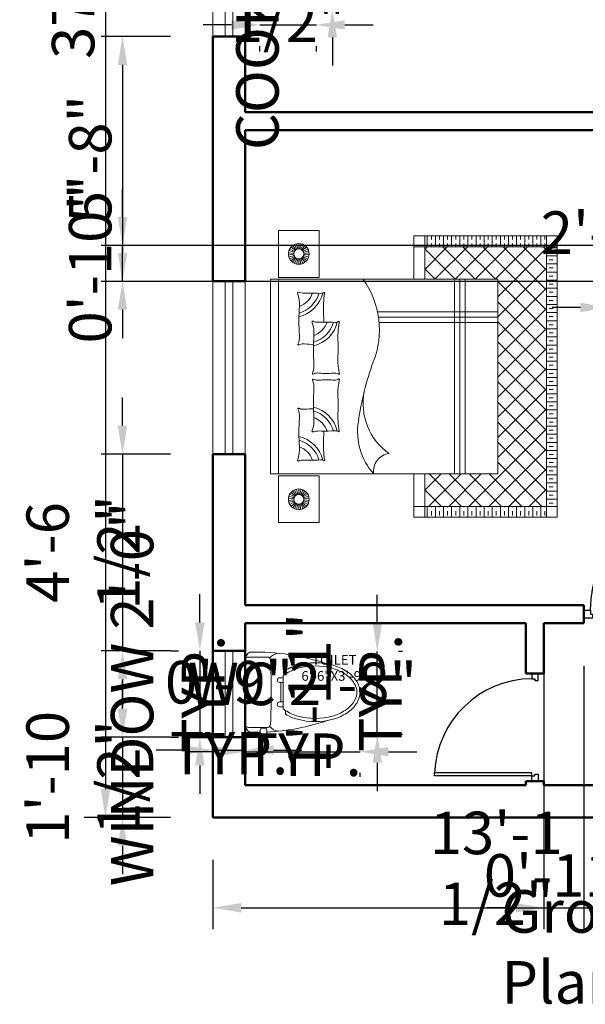
# Model space of a CAD drawing. Units: inches. Extents: x 314 to 688, y 344 to 882.
# Tile 1 of 3: x 314 to 471, y 344 to 618. Entities that reach past the tile are written whole.
import ezdxf

# ---------------------------------------------------------------- set-up
doc = ezdxf.new("R2010")
doc.units = ezdxf.units.IN
doc.header["$MEASUREMENT"] = 0
for name, color, linetype, lineweight in [('A-ANNO-TEXT', 7, 'Continuous', 25), ('A-AREA-IDEN', 7, 'Continuous', 25), ('A-DOOR', 4, 'Continuous', 25), ('A-FLOR-FIXT', 9, 'Continuous', 18), ('A-FURN', 8, 'Continuous', 18), ('WALL', 7, 'Continuous', 50), ('WINDOW', 2, 'Continuous', 18), ('YQ_DIM', 3, 'Continuous', 18)]:
    doc.layers.add(name, color=color, linetype=linetype, lineweight=lineweight)
doc.styles.add('YQ_DIM', font='SUPEROS.SHX', dxfattribs={"width": 0.8, "bigfont": 'HZDX.SHX'})
doc.dimstyles.new('yqi3_937', dxfattribs={"dimscale": 3.937008, "dimtxt": 3, "dimasz": 2, "dimexe": 1.5, "dimexo": 3, "dimgap": 0.5, "dimtad": 1, "dimdsep": 46, "dimlunit": 4, "dimtxsty": 'YQ_DIM', "dimcen": 0, "dimclrd": 256, "dimclre": 256, "dimclrt": 7, "dimadec": 1, "dimazin": 2, "dimtfac": 1, "dimtix": 1, "dimtmove": 2, "dimatfit": 2, "dimfxl": 1, "dimtolj": 1, "dimtzin": 0, "dimarcsym": 0})

# ---------------------------------------------------------------- blocks, each defined once
blk = doc.blocks.new('*D2')
at = {"layer": 'Defpoints', "color": 0, "transparency": 16777216}
for p in [(367.29, 840.23), (337.46, 396.23), (367.29, 396.23)]:
    blk.add_point(p, dxfattribs=at)
at = {"layer": 'YQ_DIM', "color": 0, "lineweight": -2, "transparency": 16777216}
for p, q in [((355.48, 840.23), (331.55, 840.23)), ((337.46, 832.36), (337.46, 404.11)), ((355.48, 396.23), (331.55, 396.23))]:
    blk.add_line(p, q, dxfattribs=at)
at = {"layer": 'YQ_DIM', "color": 0, "transparency": 16777216}
for points in [[(336.14, 832.36), (338.77, 832.36), (337.46, 840.23)], [(336.14, 404.11), (338.77, 404.11), (337.46, 396.23)]]:
    blk.add_solid(points, dxfattribs=at)
at = {"layer": 'YQ_DIM', "color": 0, "transparency": 16777216, "insert": (328.46, 618.23), "char_height": 11.811, "attachment_point": 5, "rotation": 90, "style": 'YQ_DIM'}
blk.add_mtext("\\A1;37'", dxfattribs=at)
blk = doc.blocks.new('DR_D01')
for p, q in [((-0.45, 0.93), (-0.42, 0.93)), ((-0.45, 0.03), (-0.45, 0.93)), ((-0.42, 0.03), (-0.42, 0.93)), ((-0.5, 0.03), (-0.42, 0.03)), ((-0.5, 0.03), (-0.5, -0.03)), ((-0.45, 0.03), (-0.45, 0)), ((-0.45, 0), (-0.435, 0)), ((-0.435, 0), (-0.435, -0.03)), ((0.435, 0), (0.435, -0.03)), ((0.45, 0), (0.435, 0)), ((0.45, 0.03), (0.45, 0)), ((0.5, 0.03), (0.45, 0.03)), ((0.5, -0.03), (0.5, 0.03)), ((-0.435, -0.03), (-0.5, -0.03)), ((0.435, -0.03), (0.5, -0.03))]:
    blk.add_line(p, q)
blk.add_arc((-0.4602, 0.0206), 0.9103, 0.59152, 87.46644)
blk = doc.blocks.new('WD_WIN4')
for p, q in [((-0.5, 0.5), (0.5, 0.5)), ((-0.5, 0.12), (0.5, 0.12)), ((-0.5, -0.12), (0.5, -0.12)), ((-0.5, -0.5), (0.5, -0.5))]:
    blk.add_line(p, q)
blk = doc.blocks.new('BED')
h = blk.add_hatch()
h.set_pattern_fill('TRANS', color=256, scale=12, style=0)
h.set_pattern_definition([(360, (4433.967, -9715.0492), (1e-15, 3), []), (360, (4433.967, -9713.5492), (1e-15, 3), [1.5, -1.5])])
h.paths.add_polyline_path([(48, -103), (52, -103), (52, -58), (48, -58)])
h.paths.add_polyline_path([(-48, -58), (-52, -58), (-52, -103), (-48, -103)])
h = blk.add_hatch()
h.set_pattern_fill('ANSI37', color=256, scale=42, angle=-90, style=0)
h.set_pattern_definition([(315, (7787.1367, 4477.8466), (3.7123106, 3.7123106), []), (45, (7787.1367, 4477.8466), (-3.7123106, 3.7123106), [])])
h.paths.add_polyline_path([(-36, -85), (-36, -58), (-48, -58), (-48, -103), (48, -103), (48, -58), (36, -58), (36, -85)])
h = blk.add_hatch()
h.set_pattern_fill('TRANS', color=256, scale=12, angle=-90, style=0)
h.set_pattern_definition([(270, (4433.967, -9715.0492), (3, -1e-15), []), (270, (4435.467, -9715.0492), (3, -1e-15), [1.5, -1.5])])
h.paths.add_polyline_path([(48, -107), (48, -103), (-48, -103), (-48, -107)])
for p, q in [((-36, -1), (36, -1)), ((-36, -85), (-36, -1)), ((36, -1), (36, -85)), ((-54, -4), (-54, -19)), ((-36.64, -4), (-54, -4)), ((-36.64, -4), (-36.64, -19)), ((-36, -4), (36, -4)), ((36.64, -4), (36.64, -19)), ((36.64, -4), (54, -4)), ((54, -4), (54, -19)), ((-47.19, -11.07), (-49.14, -10.66)), ((-47.07, -10.7), (-48.9, -9.89)), ((-46.88, -10.37), (-48.5, -9.2)), ((-46.62, -10.08), (-47.96, -8.6)), ((-46.31, -9.86), (-47.31, -8.13)), ((-45.96, -9.7), (-46.58, -7.8)), ((-45.58, -9.62), (-45.8, -7.63)), ((-45.2, -9.62), (-45, -7.63)), ((-44.82, -9.7), (-44.21, -7.79)), ((-44.47, -9.85), (-43.48, -8.12)), ((-44.16, -10.08), (-42.83, -8.59)), ((-43.9, -10.36), (-42.29, -9.18)), ((-43.71, -10.7), (-41.89, -9.88)), ((-43.59, -11.06), (-41.64, -10.64)), ((43.59, -11.06), (41.64, -10.64)), ((43.71, -10.7), (41.89, -9.88)), ((43.9, -10.36), (42.29, -9.18)), ((44.16, -10.08), (42.83, -8.59)), ((44.47, -9.85), (43.48, -8.12)), ((44.82, -9.7), (44.21, -7.79)), ((45.2, -9.62), (45, -7.63)), ((45.58, -9.62), (45.8, -7.63)), ((45.96, -9.7), (46.58, -7.8)), ((46.31, -9.86), (47.31, -8.13)), ((46.62, -10.08), (47.96, -8.6)), ((46.88, -10.37), (48.5, -9.2)), ((47.07, -10.7), (48.9, -9.89)), ((47.19, -11.07), (49.14, -10.66)), ((-47.23, -11.45), (-49.23, -11.45)), ((-47.19, -11.83), (-49.14, -12.25)), ((-47.07, -12.2), (-48.89, -13.01)), ((-46.87, -12.53), (-48.49, -13.71)), ((-46.62, -12.81), (-47.95, -14.3)), ((-46.3, -13.04), (-47.3, -14.77)), ((-45.95, -13.2), (-46.57, -15.1)), ((-45.58, -13.27), (-45.78, -15.26)), ((-45.19, -13.27), (-44.98, -15.26)), ((-44.82, -13.19), (-44.2, -15.09)), ((-44.47, -13.04), (-43.46, -14.77)), ((-44.16, -12.81), (-42.82, -14.29)), ((-43.9, -12.52), (-42.28, -13.7)), ((-43.71, -12.19), (-41.88, -13)), ((-43.59, -11.83), (-41.63, -12.24)), ((-43.55, -11.44), (-41.55, -11.44)), ((43.55, -11.44), (41.55, -11.44)), ((43.59, -11.83), (41.63, -12.24)), ((43.71, -12.19), (41.88, -13)), ((43.9, -12.52), (42.28, -13.7)), ((44.16, -12.81), (42.82, -14.29)), ((44.47, -13.04), (43.46, -14.77)), ((44.82, -13.19), (44.2, -15.09)), ((45.19, -13.27), (44.98, -15.26)), ((45.58, -13.27), (45.78, -15.26)), ((45.95, -13.2), (46.57, -15.1)), ((46.3, -13.04), (47.3, -14.77)), ((46.62, -12.81), (47.95, -14.3)), ((46.87, -12.53), (48.49, -13.71)), ((47.07, -12.2), (48.89, -13.01)), ((47.19, -11.83), (49.14, -12.25)), ((47.23, -11.45), (49.23, -11.45)), ((-36.64, -19), (-54, -19)), ((36.64, -19), (54, -19)), ((20, -85), (20, -41.14)), ((22, -85), (22, -40.91)), ((24, -85), (24, -40.55)), ((-52, -54), (-52, -107)), ((-52, -54), (-36, -54)), ((-48, -54), (-48, -107)), ((36, -54), (52, -54)), ((48, -54), (48, -107)), ((52, -54), (52, -107)), ((-52, -58), (-36, -58)), ((36, -58), (52, -58)), ((36, -69), (-36, -69)), ((36, -71), (-36, -71)), ((36, -73), (-36, -73)), ((36, -85), (-36, -85)), ((-52, -103), (52, -103)), ((-52, -107), (52, -107))]:
    blk.add_line(p, q)
for centre, radius in [((-45.39, -11.45), 3.84), ((-45.39, -11.45), 1.84), ((45.39, -11.45), 3.84), ((45.39, -11.45), 1.84)]:
    blk.add_circle(centre, radius)
for centre, radius, start, end in [((-30.92, -11.24), 0.328, 35.8976, 208.6272), ((30.92, -11.24), 0.328, 331.3728, 144.1024), ((-42.38, -17.5), 12.73, 27.1629, 28.6272), ((-44.37, -13.89), 13.5, 357.4804, 9.3956), ((10.15, -16.29), 41.07, 177.4804, 184.5075), ((-33.8, -8.61), 8.46, 289.8695, 338.9843), ((-33.8, -8.61), 12.06, 283.8498, 346.0842), ((-33.8, -8.61), 10.71, 286.0319, 344.1205), ((-26.84, 0.13), 11.82, 251.1782, 273.3982), ((-20.92, -99.64), 88.13, 86.2964, 93.3982), ((-14.79, -4.98), 6.73, 266.2964, 294.303), ((-8.24, -13.16), 3.86, 159.0146, 186.273), ((-36.64, -16.28), 24.71, 358.5721, 6.273), ((-11.92, -11.33), 0.242, 335.7259, 114.303), ((-5.69, -14.14), 6.59, 155.7259, 159.0146), ((11.92, -11.33), 0.242, 65.697, 204.2741), ((5.69, -14.14), 6.59, 20.9854, 24.2741), ((8.24, -13.16), 3.86, 353.727, 20.9854), ((36.64, -16.28), 24.71, 173.727, 181.4279), ((14.79, -4.98), 6.73, 245.697, 273.7036), ((20.92, -99.64), 88.13, 86.6018, 93.7036), ((33.8, -8.61), 12.06, 193.9158, 256.1502), ((33.8, -8.61), 10.71, 195.8795, 253.9681), ((33.8, -8.61), 8.46, 201.0157, 250.1305), ((26.84, 0.13), 11.82, 266.6018, 288.8218), ((-10.15, -16.29), 41.07, 355.4925, 2.5196), ((44.37, -13.89), 13.5, 170.6044, 182.5196), ((42.38, -17.5), 12.73, 151.3728, 152.8371), ((-20.16, -16.62), 0.328, 35.8976, 208.6272), ((-31.62, -22.87), 12.73, 27.1629, 28.6272), ((-33.61, -19.26), 13.5, 357.4804, 9.3956), ((-23.04, -13.99), 8.46, 289.8695, 338.9843), ((-23.04, -13.99), 12.06, 283.8498, 346.0842), ((-23.04, -13.99), 10.71, 286.0319, 344.1205), ((-16.08, -5.24), 11.82, 251.1782, 273.3982), ((-10.15, -105.01), 88.13, 86.2964, 93.3982), ((-4.03, -10.35), 6.73, 266.2964, 294.303), ((2.52, -18.53), 3.86, 159.0146, 186.273), ((-1.16, -16.7), 0.242, 335.7259, 114.303), ((5.07, -19.51), 6.59, 155.7259, 159.0146), ((1.16, -16.7), 0.242, 65.697, 204.2741), ((-5.07, -19.51), 6.59, 20.9854, 24.2741), ((-2.52, -18.53), 3.86, 353.727, 20.9854), ((4.03, -10.35), 6.73, 245.697, 273.7036), ((10.15, -105.01), 88.13, 86.6018, 93.7036), ((23.04, -13.99), 12.06, 193.9158, 256.1502), ((23.04, -13.99), 10.71, 195.8795, 253.9681), ((23.04, -13.99), 8.46, 201.0157, 250.1305), ((16.08, -5.24), 11.82, 266.6018, 288.8218), ((20.16, -16.62), 0.328, 331.3728, 144.1024), ((33.61, -19.26), 13.5, 170.6044, 182.5196), ((31.62, -22.87), 12.73, 151.3728, 152.8371), ((-30.88, -20.82), 0.25, 147.6219, 311.9343), ((-32.72, -19.65), 1.93, 327.6219, 339.2246), ((-32.67, -19.67), 1.88, 339.2246, 4.5075), ((-25.16, -53.53), 33, 93.5164, 99.6766), ((-25.27, -51.86), 31.33, 86.4836, 93.5164), ((-21.12, 15.68), 36.34, 266.4836, 271.5234), ((20.91, -21.66), 41.07, 177.4804, 184.5075), ((-25.88, -21.66), 24.71, 354.3784, 6.273), ((25.88, -21.66), 24.71, 173.727, 185.6216), ((-20.91, -21.66), 41.07, 355.4925, 2.5196), ((21.12, 15.68), 36.34, 268.4766, 273.5164), ((25.27, -51.86), 31.33, 86.4836, 93.5164), ((25.16, -53.53), 33, 80.3234, 86.4836), ((30.88, -20.82), 0.25, 228.0657, 32.3781), ((32.67, -19.67), 1.88, 175.4925, 200.7754), ((32.72, -19.65), 1.93, 200.7754, 212.3781), ((-21.91, -25.04), 1.88, 339.2246, 4.5075), ((2.55, -24.46), 3.86, 174.3784, 204.7617), ((-2.55, -24.46), 3.86, 335.2383, 5.6216), ((21.91, -25.04), 1.88, 175.4925, 200.7754), ((-20.12, -26.19), 0.25, 147.6219, 311.9343), ((-21.96, -25.02), 1.93, 327.6219, 339.2246), ((-14.4, -58.9), 33, 93.5164, 99.6766), ((-14.51, -57.23), 31.33, 86.4836, 93.5164), ((-10.35, 10.3), 36.34, 266.4836, 275.306), ((-5.78, -38.98), 13.15, 77.9645, 95.306), ((2.5, -0.17), 26.53, 257.9645, 261.9243), ((-1.09, -26.25), 0.228, 231.9005, 52.8902), ((1.09, -26.25), 0.228, 127.1098, 308.0995), ((-2.5, -0.17), 26.53, 278.0757, 282.0355), ((5.78, -38.98), 13.15, 84.694, 102.0355), ((10.35, 10.3), 36.34, 264.694, 273.5164), ((14.51, -57.23), 31.33, 86.4836, 93.5164), ((14.4, -58.9), 33, 80.3234, 86.4836), ((20.12, -26.19), 0.25, 228.0657, 32.3781), ((21.96, -25.02), 1.93, 200.7754, 212.3781), ((-20.27, -56.85), 23.66, 81.0857, 131.6581), ((-9.91, -57.83), 22.61, 78.6456, 145.1521), ((-32.56, -143.87), 111.55, 70.0977, 81.7735), ((17.27, -9.21), 32.05, 248.2778, 305.7663), ((-34.97, -45.63), 6.55, 6.3172, 99.0807)]:
    blk.add_arc(centre, radius, start, end)
blk = doc.blocks.new('yq_matong_01')
for p, q in [((0, 200.5), (0, -200.5)), ((20, 220.5), (138.8, 220.5)), ((252.5, 138), (252.5, 114.5)), ((215.8, 91), (238, 91)), ((238, 104.1), (238, -104.1)), ((215.8, 61), (238, 61)), ((223, 61), (223, -61)), ((215.8, -61), (238, -61)), ((215.8, -91), (238, -91)), ((252.5, -114.5), (252.5, -138)), ((20, -220.5), (138.8, -220.5)), ((97.4, -220.5), (97.4, -225.5)), ((97.4, -225.5), (131.6, -225.5)), ((131.6, -220.5), (131.6, -225.5))]:
    blk.add_line(p, q)
for centre, radius, start, end in [((54.8, 202.4), 54.8, 117.32201, 181.89921), ((63.9, -1165.4), 1416.8, 71.40679, 91.38565), ((20, 200.5), 20, 90, 180), ((138.8, 200.5), 20, 2.30634, 90), ((216.6, 161.2), 83.2, 95.49628, 139.93242), ((-4840.4, 0), 5003.3, 357.69366, 2.30634), ((406.6, -122.9), 283, 105.20877, 123.27785), ((406.6, -122.9), 303, 105.20877, 120.56985), ((439, -242.2), 426.7, 74.79123, 105.20877), ((439, -242.2), 406.7, 74.79123, 105.20877), ((471.4, -122.9), 283, 56.72215, 74.79123), ((471.4, -122.9), 303, 56.72215, 74.79123), ((520.9, -47.5), 212.8, 32.25649, 56.72215), ((215.8, 76), 15, 90, 270), ((357.1, -47.5), 192.8, 123.27785, 128.13838), ((520.9, -47.5), 192.8, 32.25649, 56.72215), ((596.2, 0), 123.8, 360, 32.25649), ((596.2, 0), 103.8, 360, 32.25649), ((215.8, -76), 15, 90, 270), ((520.9, 47.5), 192.8, 303.27785, 327.74351), ((596.2, 0), 103.8, 327.74351, 360), ((596.2, 0), 123.8, 327.74351, 360), ((357.1, 47.5), 192.8, 231.86162, 236.72215), ((406.6, 122.9), 283, 236.72215, 254.79123), ((471.4, 122.9), 283, 285.20877, 303.27785), ((520.9, 47.5), 212.8, 303.27785, 327.74351), ((63.9, 1165.4), 1416.8, 272.89667, 288.59321), ((406.6, 122.9), 303, 239.43015, 254.79123), ((439, 242.2), 426.7, 254.79123, 285.20877), ((439, 242.2), 406.7, 254.79123, 285.20877), ((471.4, 122.9), 303, 285.20877, 303.27785), ((51.3, -204.4), 51.4, 175.68696, 245.09182), ((20, -200.5), 20, 180, 270), ((156.6, -247.4), 63.1, 159.68336, 188.49388), ((72.4, -247.4), 63.1, 352.09441, 20.31664), ((138.8, -200.5), 20, 270, 357.69366), ((216.6, -161.2), 83.2, 220.06758, 264.50372), ((63.9, 1165.4), 1416.8, 268.61435, 271.20362), ((114.1, -225.6), 37, 237.52867, 304.27722)]:
    blk.add_arc(centre, radius, start, end)
blk = doc.blocks.new('*D18')
at = {"layer": 'Defpoints', "color": 0, "transparency": 16777216}
for p in [(367.29, 442.57), (363.69, 418.57), (367.29, 418.57)]:
    blk.add_point(p, dxfattribs=at)
at = {"layer": 'YQ_DIM', "lineweight": -2, "transparency": 16777216}
for p, q in [((363.69, 450.44), (363.69, 458.32)), ((355.48, 442.57), (357.79, 442.57)), ((363.69, 442.57), (363.69, 418.57)), ((355.48, 418.57), (357.79, 418.57)), ((363.69, 410.69), (363.69, 402.82))]:
    blk.add_line(p, q, dxfattribs=at)
at = {"layer": 'YQ_DIM', "transparency": 16777216}
for points in [[(362.38, 450.44), (365.01, 450.44), (363.69, 442.57)], [(362.38, 410.69), (365.01, 410.69), (363.69, 418.57)]]:
    blk.add_solid(points, dxfattribs=at)
at = {"layer": 'YQ_DIM', "color": 7, "transparency": 16777216, "insert": (354.7, 430.57), "char_height": 11.811, "attachment_point": 5, "rotation": 90, "style": 'YQ_DIM'}
blk.add_mtext('\\A1;WINDOW 2\'-0" TYP.', dxfattribs=at)
blk = doc.blocks.new('*D19')
at = {"layer": 'Defpoints', "color": 0, "transparency": 16777216}
for p in [(367.29, 418.57), (376.29, 418.57), (376.29, 414.97)]:
    blk.add_point(p, dxfattribs=at)
at = {"layer": 'YQ_DIM', "lineweight": -2, "transparency": 16777216}
for p, q in [((359.42, 414.97), (351.55, 414.97)), ((367.29, 414.97), (376.29, 414.97)), ((384.17, 414.97), (392.04, 414.97)), ((367.29, 406.76), (367.29, 409.06)), ((376.29, 406.76), (376.29, 409.06))]:
    blk.add_line(p, q, dxfattribs=at)
at = {"layer": 'YQ_DIM', "transparency": 16777216}
for points in [[(359.42, 416.28), (359.42, 413.66), (367.29, 414.97)], [(384.17, 416.28), (384.17, 413.66), (376.29, 414.97)]]:
    blk.add_solid(points, dxfattribs=at)
at = {"layer": 'YQ_DIM', "color": 7, "transparency": 16777216, "insert": (371.79, 423.97), "char_height": 11.811, "attachment_point": 5, "style": 'YQ_DIM'}
blk.add_mtext('\\A1;0\'-9" TYP.', dxfattribs=at)
blk = doc.blocks.new('*D25')
at = {"layer": 'Defpoints', "color": 0, "transparency": 16777216}
for p in [(477.31, 543.36), (511.87, 543.36), (477.31, 537.96)]:
    blk.add_point(p, dxfattribs=at)
at = {"layer": 'YQ_DIM', "lineweight": -2, "transparency": 16777216}
for p, q in [((469.44, 537.96), (461.57, 537.96)), ((511.87, 537.96), (477.31, 537.96)), ((519.75, 537.96), (527.62, 537.96)), ((477.31, 531.55), (477.31, 532.05)), ((511.87, 531.55), (511.87, 532.05))]:
    blk.add_line(p, q, dxfattribs=at)
at = {"layer": 'YQ_DIM', "transparency": 16777216}
for points in [[(469.44, 539.27), (469.44, 536.65), (477.31, 537.96)], [(519.75, 539.27), (519.75, 536.65), (511.87, 537.96)]]:
    blk.add_solid(points, dxfattribs=at)
at = {"layer": 'YQ_DIM', "color": 7, "transparency": 16777216, "insert": (494.59, 548.93), "char_height": 11.811, "attachment_point": 5, "style": 'YQ_DIM'}
blk.add_mtext('\\A1;2\'-10 1/2" TYP.', dxfattribs=at)
blk = doc.blocks.new('*D28')
at = {"layer": 'Defpoints', "color": 0, "transparency": 16777216}
for p in [(376.22, 419.31), (408.2, 419.31), (408.2, 414.52)]:
    blk.add_point(p, dxfattribs=at)
at = {"layer": 'YQ_DIM', "lineweight": -2, "transparency": 16777216}
for p, q in [((368.35, 414.52), (360.47, 414.52)), ((376.22, 414.52), (408.2, 414.52)), ((416.07, 414.52), (423.95, 414.52)), ((376.22, 407.5), (376.22, 408.61)), ((408.2, 407.5), (408.2, 408.61))]:
    blk.add_line(p, q, dxfattribs=at)
at = {"layer": 'YQ_DIM', "transparency": 16777216}
for points in [[(368.35, 415.83), (368.35, 413.21), (376.22, 414.52)], [(416.07, 415.83), (416.07, 413.21), (408.2, 414.52)]]:
    blk.add_solid(points, dxfattribs=at)
at = {"layer": 'YQ_DIM', "color": 7, "transparency": 16777216, "insert": (392.21, 423.52), "char_height": 11.811, "attachment_point": 5, "style": 'YQ_DIM'}
blk.add_mtext('\\A1;WC 2\'-8" TYP.', dxfattribs=at)
blk = doc.blocks.new('*D29')
at = {"layer": 'Defpoints', "color": 0, "transparency": 16777216}
for p in [(408.2, 442.34), (412.99, 442.34), (408.2, 419.31)]:
    blk.add_point(p, dxfattribs=at)
at = {"layer": 'YQ_DIM', "lineweight": -2, "transparency": 16777216}
for p, q in [((412.99, 450.22), (412.99, 458.09)), ((412.99, 419.31), (412.99, 442.34)), ((420.01, 442.34), (418.9, 442.34)), ((420.01, 419.31), (418.9, 419.31)), ((412.99, 411.44), (412.99, 403.57))]:
    blk.add_line(p, q, dxfattribs=at)
at = {"layer": 'YQ_DIM', "transparency": 16777216}
for points in [[(411.68, 450.22), (414.31, 450.22), (412.99, 442.34)], [(411.68, 411.44), (414.31, 411.44), (412.99, 419.31)]]:
    blk.add_solid(points, dxfattribs=at)
at = {"layer": 'YQ_DIM', "color": 7, "transparency": 16777216, "insert": (404, 430.83), "char_height": 11.811, "attachment_point": 5, "rotation": 90, "style": 'YQ_DIM'}
blk.add_mtext('\\A1;1\'-11" TYP.', dxfattribs=at)
blk = doc.blocks.new('*D30')
at = {"layer": 'Defpoints', "color": 0, "transparency": 16777216}
for p in [(396.07, 650.46), (400.5, 650.46), (396.07, 620.93)]:
    blk.add_point(p, dxfattribs=at)
at = {"layer": 'YQ_DIM', "lineweight": -2, "transparency": 16777216}
for p, q in [((400.5, 658.33), (400.5, 666.2)), ((400.5, 620.93), (400.5, 650.46)), ((407.88, 650.46), (406.41, 650.46)), ((407.88, 620.93), (406.41, 620.93)), ((400.5, 613.05), (400.5, 605.18))]:
    blk.add_line(p, q, dxfattribs=at)
at = {"layer": 'YQ_DIM', "transparency": 16777216}
for points in [[(399.19, 658.33), (401.81, 658.33), (400.5, 650.46)], [(399.19, 613.05), (401.81, 613.05), (400.5, 620.93)]]:
    blk.add_solid(points, dxfattribs=at)
at = {"layer": 'YQ_DIM', "color": 7, "transparency": 16777216, "insert": (389.53, 635.69), "char_height": 11.811, "attachment_point": 5, "rotation": 90, "style": 'YQ_DIM'}
blk.add_mtext('\\A1;COOKTOP 2\'-5 1/2"', dxfattribs=at)
blk = doc.blocks.new('*D31')
at = {"layer": 'Defpoints', "color": 0, "transparency": 16777216}
for p in [(380.33, 620.93), (396.07, 620.93), (396.07, 616.5)]:
    blk.add_point(p, dxfattribs=at)
at = {"layer": 'YQ_DIM', "lineweight": -2, "transparency": 16777216}
for p, q in [((372.45, 616.5), (364.58, 616.5)), ((380.33, 616.5), (396.07, 616.5)), ((403.95, 616.5), (411.82, 616.5)), ((380.33, 609.12), (380.33, 610.59)), ((396.07, 609.12), (396.07, 610.59))]:
    blk.add_line(p, q, dxfattribs=at)
at = {"layer": 'YQ_DIM', "transparency": 16777216}
for points in [[(372.45, 617.81), (372.45, 615.19), (380.33, 616.5)], [(403.95, 617.81), (403.95, 615.19), (396.07, 616.5)]]:
    blk.add_solid(points, dxfattribs=at)
at = {"layer": 'YQ_DIM', "color": 7, "transparency": 16777216, "insert": (388.2, 627.47), "char_height": 11.811, "attachment_point": 5, "style": 'YQ_DIM'}
blk.add_mtext('\\A1;1\'-3 1/2"', dxfattribs=at)
blk = doc.blocks.new('*D40')
at = {"layer": 'Defpoints', "color": 0, "transparency": 16777216}
for p in [(342.19, 555.23), (607.29, 555.23), (607.29, 545.23)]:
    blk.add_point(p, dxfattribs=at)
at = {"layer": 'YQ_DIM', "lineweight": -2, "transparency": 16777216}
for p, q in [((342.19, 563.11), (342.19, 570.98)), ((595.48, 555.23), (336.29, 555.23)), ((342.19, 545.23), (342.19, 555.23)), ((595.48, 545.23), (336.29, 545.23)), ((342.19, 537.36), (342.19, 529.48))]:
    blk.add_line(p, q, dxfattribs=at)
at = {"layer": 'YQ_DIM', "transparency": 16777216}
for points in [[(340.88, 563.11), (343.51, 563.11), (342.19, 555.23)], [(340.88, 537.36), (343.51, 537.36), (342.19, 545.23)]]:
    blk.add_solid(points, dxfattribs=at)
at = {"layer": 'YQ_DIM', "color": 7, "transparency": 16777216, "insert": (333.2, 550.23), "char_height": 11.811, "attachment_point": 5, "rotation": 90, "style": 'YQ_DIM'}
blk.add_mtext('\\A1;0\'-10"', dxfattribs=at)
blk = doc.blocks.new('*D43')
at = {"layer": 'Defpoints', "color": 0, "transparency": 16777216}
for p in [(367.29, 613.23), (342.19, 545.23), (367.29, 545.23)]:
    blk.add_point(p, dxfattribs=at)
at = {"layer": 'YQ_DIM', "lineweight": -2, "transparency": 16777216}
for p, q in [((355.48, 613.23), (336.29, 613.23)), ((342.19, 605.36), (342.19, 553.11)), ((355.48, 545.23), (336.29, 545.23))]:
    blk.add_line(p, q, dxfattribs=at)
at = {"layer": 'YQ_DIM', "transparency": 16777216}
for points in [[(340.88, 605.36), (343.51, 605.36), (342.19, 613.23)], [(340.88, 553.11), (343.51, 553.11), (342.19, 545.23)]]:
    blk.add_solid(points, dxfattribs=at)
at = {"layer": 'YQ_DIM', "color": 7, "transparency": 16777216, "insert": (333.2, 579.23), "char_height": 11.811, "attachment_point": 5, "rotation": 90, "style": 'YQ_DIM'}
blk.add_mtext('\\A1;5\'-8"', dxfattribs=at)
blk = doc.blocks.new('*D44')
at = {"layer": 'Defpoints', "color": 0, "transparency": 16777216}
for p in [(367.29, 497.23), (342.19, 442.57), (367.29, 442.57)]:
    blk.add_point(p, dxfattribs=at)
at = {"layer": 'YQ_DIM', "lineweight": -2, "transparency": 16777216}
for p, q in [((342.19, 505.11), (342.19, 512.98)), ((355.48, 497.23), (336.29, 497.23)), ((342.19, 497.23), (342.19, 442.57)), ((355.48, 442.57), (336.29, 442.57)), ((342.19, 434.69), (342.19, 426.82))]:
    blk.add_line(p, q, dxfattribs=at)
at = {"layer": 'YQ_DIM', "transparency": 16777216}
for points in [[(340.88, 505.11), (343.51, 505.11), (342.19, 497.23)], [(340.88, 434.69), (343.51, 434.69), (342.19, 442.57)]]:
    blk.add_solid(points, dxfattribs=at)
at = {"layer": 'YQ_DIM', "color": 7, "transparency": 16777216, "insert": (331.23, 469.9), "char_height": 11.811, "attachment_point": 5, "rotation": 90, "style": 'YQ_DIM'}
blk.add_mtext('\\A1;4\'-6 1/2"', dxfattribs=at)
blk = doc.blocks.new('*D45')
at = {"layer": 'Defpoints', "color": 0, "transparency": 16777216}
for p in [(367.29, 418.57), (342.19, 396.23), (367.29, 396.23)]:
    blk.add_point(p, dxfattribs=at)
at = {"layer": 'YQ_DIM', "lineweight": -2, "transparency": 16777216}
for p, q in [((342.19, 426.44), (342.19, 434.32)), ((355.48, 418.57), (336.29, 418.57)), ((342.19, 418.57), (342.19, 396.23)), ((355.48, 396.23), (336.29, 396.23)), ((342.19, 388.36), (342.19, 380.48))]:
    blk.add_line(p, q, dxfattribs=at)
at = {"layer": 'YQ_DIM', "transparency": 16777216}
for points in [[(340.88, 426.44), (343.51, 426.44), (342.19, 418.57)], [(340.88, 388.36), (343.51, 388.36), (342.19, 396.23)]]:
    blk.add_solid(points, dxfattribs=at)
at = {"layer": 'YQ_DIM', "color": 7, "transparency": 16777216, "insert": (331.23, 407.4), "char_height": 11.811, "attachment_point": 5, "rotation": 90, "style": 'YQ_DIM'}
blk.add_mtext('\\A1;1\'-10 1/2"', dxfattribs=at)
blk = doc.blocks.new('*D46')
at = {"layer": 'Defpoints', "color": 0, "transparency": 16777216}
for p in [(367.29, 396.23), (524.79, 396.23), (524.79, 371.13)]:
    blk.add_point(p, dxfattribs=at)
at = {"layer": 'YQ_DIM', "lineweight": -2, "transparency": 16777216}
for p, q in [((367.29, 384.42), (367.29, 365.23)), ((524.79, 384.42), (524.79, 365.23)), ((375.17, 371.13), (516.92, 371.13))]:
    blk.add_line(p, q, dxfattribs=at)
at = {"layer": 'YQ_DIM', "transparency": 16777216}
for points in [[(375.17, 372.44), (375.17, 369.82), (367.29, 371.13)], [(516.92, 372.44), (516.92, 369.82), (524.79, 371.13)]]:
    blk.add_solid(points, dxfattribs=at)
at = {"layer": 'YQ_DIM', "color": 7, "transparency": 16777216, "insert": (446.04, 382.1), "char_height": 11.811, "attachment_point": 5, "style": 'YQ_DIM'}
blk.add_mtext('\\A1;13\'-1 1/2"', dxfattribs=at)
blk = doc.blocks.new('*D53')
at = {"layer": 'Defpoints', "color": 0, "transparency": 16777216}
for p in [(459.29, 450.23), (470.42, 450.23), (470.42, 371.13)]:
    blk.add_point(p, dxfattribs=at)
at = {"layer": 'YQ_DIM', "lineweight": -2, "transparency": 16777216}
for p, q in [((459.29, 438.42), (459.29, 365.23)), ((470.42, 438.42), (470.42, 365.23)), ((451.42, 371.13), (443.55, 371.13)), ((459.29, 371.13), (470.42, 371.13)), ((478.29, 371.13), (486.17, 371.13))]:
    blk.add_line(p, q, dxfattribs=at)
at = {"layer": 'YQ_DIM', "transparency": 16777216}
for points in [[(451.42, 372.44), (451.42, 369.82), (459.29, 371.13)], [(478.29, 372.44), (478.29, 369.82), (470.42, 371.13)]]:
    blk.add_solid(points, dxfattribs=at)
at = {"layer": 'YQ_DIM', "color": 7, "transparency": 16777216, "insert": (464.86, 380.13), "char_height": 11.811, "attachment_point": 5, "style": 'YQ_DIM'}
blk.add_mtext('\\A1;0\'-11"', dxfattribs=at)

msp = doc.modelspace()

# ---------------------------------------------------------------- linework, layer by layer
at = {"layer": 'WALL'}
for p, q in [((367.294, 545.233), (367.294, 613.233)), ((376.294, 613.233), (367.294, 613.233)), ((376.294, 592.233), (376.294, 613.233)), ((376.294, 592.233), (513.294, 592.233)), ((376.294, 587.233), (508.294, 587.233)), ((376.294, 545.233), (376.294, 587.233)), ((376.294, 545.233), (367.294, 545.233)), ((367.294, 396.233), (367.294, 497.233)), ((376.294, 497.233), (367.294, 497.233)), ((376.294, 455.233), (376.294, 497.233)), ((376.294, 455.233), (470.42, 455.233)), ((470.42, 455.233), (470.42, 450.233)), ((376.294, 450.233), (454.294, 450.233)), ((376.294, 450.233), (376.294, 405.233)), ((454.294, 450.233), (454.294, 436.285)), ((459.294, 450.233), (459.294, 436.285)), ((459.294, 450.233), (470.42, 450.233)), ((367.294, 442.569), (376.294, 442.569)), ((454.294, 436.285), (459.294, 436.285)), ((367.294, 418.569), (376.294, 418.569)), ((376.294, 405.233), (454.294, 405.233)), ((454.294, 406.285), (459.294, 406.285)), ((454.294, 406.285), (454.294, 405.233)), ((459.294, 406.285), (459.294, 405.233)), ((459.294, 405.233), (563.294, 405.233)), ((367.294, 396.233), (524.794, 396.233))]:
    msp.add_line(p, q, dxfattribs=at)

# ---------------------------------------------------------------- block references
at = {"layer": 'A-DOOR', "xscale": -36, "yscale": 36, "zscale": 36}
msp.add_blockref('DR_D01', (488.42, 452.733), dxfattribs=at)
at = {"layer": 'A-DOOR', "xscale": 30, "yscale": 30, "zscale": 30, "rotation": 90}
msp.add_blockref('DR_D01', (456.794, 421.285), dxfattribs=at)
at = {"layer": 'A-FLOR-FIXT', "xscale": 0.0443114336064022, "yscale": 0.0443114336064022, "zscale": 0.0443114336064022}
msp.add_blockref('yq_matong_01', (376.294, 431.044), dxfattribs=at)
at = {"layer": 'A-FURN', "xscale": 0.7515029440786926, "yscale": 0.7515029440786926, "zscale": 0.7515029440786926, "rotation": 90}
msp.add_blockref('BED', (382.57, 518.754), dxfattribs=at)
at = {"layer": 'WINDOW'}
for p, xscale, yscale, zscale, rotation in [((371.794, 631.233), 36, 8.999999999999657, 36, 269.9999999999997), ((371.794, 521.233), 48, 9.000000000000966, 48, 269.9999999999997), ((371.794, 430.569), 24, 9.000000000000227, 24, 269.9999999999998)]:
    msp.add_blockref('WD_WIN4', p, dxfattribs=dict(at, xscale=xscale, yscale=yscale, zscale=zscale, rotation=rotation))

# ---------------------------------------------------------------- texts
at = {"layer": 'A-ANNO-TEXT', "insert": (447.466, 376.019), "char_height": 11.81102, "width": 110.27862, "attachment_point": 1, "style": 'YQ_DIM'}
msp.add_mtext('Ground Floor Plan', dxfattribs=at)
at = {"layer": 'A-AREA-IDEN', "insert": (390.498, 441.398), "char_height": 2.69012, "width": 21.10895, "attachment_point": 1, "style": 'YQ_DIM'}
msp.add_mtext('\\pxqc;TOILET\\P6\'-6"X3\'-9"', dxfattribs=at)

# ---------------------------------------------------------------- dimensions: what is measured, and where the dimension line sits
at = {"layer": 'YQ_DIM'}
dim = msp.add_aligned_dim(p1=(367.294, 840.233), p2=(367.294, 396.233), distance=-29.838, dimstyle='yqi3_937', override={"dimclrd": 0, "dimclre": 0, "dimclrt": 0}, dxfattribs=at)
dim.commit()
dim.dimension.update_dxf_attribs({"geometry": '*D2', "text_midpoint": (328.457, 618.233)})
for base, p1, p2, angle, text, picture, middle in [((400.502, 650.456), (396.073, 620.929), (396.073, 650.456), 90, 'COOKTOP <>', '*D30', (389.535, 635.693)), ((477.314, 537.959), (511.874, 543.359), (477.314, 543.359), 180, '<> TYP.', '*D25', (494.594, 548.926)), ((363.694, 418.569), (367.294, 442.569), (367.294, 418.569), 270, 'WINDOW <> TYP.', '*D18', (354.695, 430.569)), ((412.995, 442.344), (408.198, 419.315), (408.198, 442.344), 90, '<> TYP.', '*D29', (403.996, 430.829))]:
    dim = msp.add_linear_dim(base=base, p1=p1, p2=p2, angle=angle, text=text, dimstyle='yqi3_937', override={"dimdec": 1, "dimlfac": 1, "dimrnd": 0, "dimzin": 1, "dimdsep": 46, "dimlunit": 4, "dimfrac": 2}, dxfattribs=at)
    dim.commit()
    dim.dimension.update_dxf_attribs({"geometry": picture, "text_midpoint": middle})
for base, p1, p2, picture, middle in [((396.073, 616.5), (380.325, 620.929), (396.073, 620.929), '*D31', (388.199, 627.467)), ((470.42, 371.133), (459.294, 450.233), (470.42, 450.233), '*D53', (464.857, 380.131)), ((524.794, 371.133), (367.294, 396.233), (524.794, 396.233), '*D46', (446.044, 382.1))]:
    dim = msp.add_linear_dim(base=base, p1=p1, p2=p2, dimstyle='yqi3_937', override={"dimdec": 1, "dimlfac": 1, "dimrnd": 0, "dimzin": 1, "dimdsep": 46, "dimlunit": 4, "dimfrac": 2}, dxfattribs=at)
    dim.commit()
    dim.dimension.update_dxf_attribs({"geometry": picture, "text_midpoint": middle})
for base, p1, p2, picture, middle in [((342.194, 545.233), (367.294, 613.233), (367.294, 545.233), '*D43', (333.195, 579.233)), ((342.194, 555.233), (607.294, 545.233), (607.294, 555.233), '*D40', (333.195, 550.233)), ((342.194, 442.569), (367.294, 497.233), (367.294, 442.569), '*D44', (331.227, 469.901)), ((342.194, 396.233), (367.294, 418.569), (367.294, 396.233), '*D45', (331.227, 407.401))]:
    dim = msp.add_linear_dim(base=base, p1=p1, p2=p2, angle=90, dimstyle='yqi3_937', override={"dimdec": 1, "dimlfac": 1, "dimrnd": 0, "dimzin": 1, "dimdsep": 46, "dimlunit": 4, "dimfrac": 2}, dxfattribs=at)
    dim.commit()
    dim.dimension.update_dxf_attribs({"geometry": picture, "text_midpoint": middle})
for base, p1, p2, text, picture, middle in [((408.198, 414.518), (376.223, 419.315), (408.198, 419.315), 'WC <> TYP.', '*D28', (392.21, 423.517)), ((376.294, 414.969), (367.294, 418.569), (376.294, 418.569), '<> TYP.', '*D19', (371.794, 423.968))]:
    dim = msp.add_linear_dim(base=base, p1=p1, p2=p2, text=text, dimstyle='yqi3_937', override={"dimdec": 1, "dimlfac": 1, "dimrnd": 0, "dimzin": 1, "dimdsep": 46, "dimlunit": 4, "dimfrac": 2}, dxfattribs=at)
    dim.commit()
    dim.dimension.update_dxf_attribs({"geometry": picture, "text_midpoint": middle})

doc.saveas('drawing.dxf')
